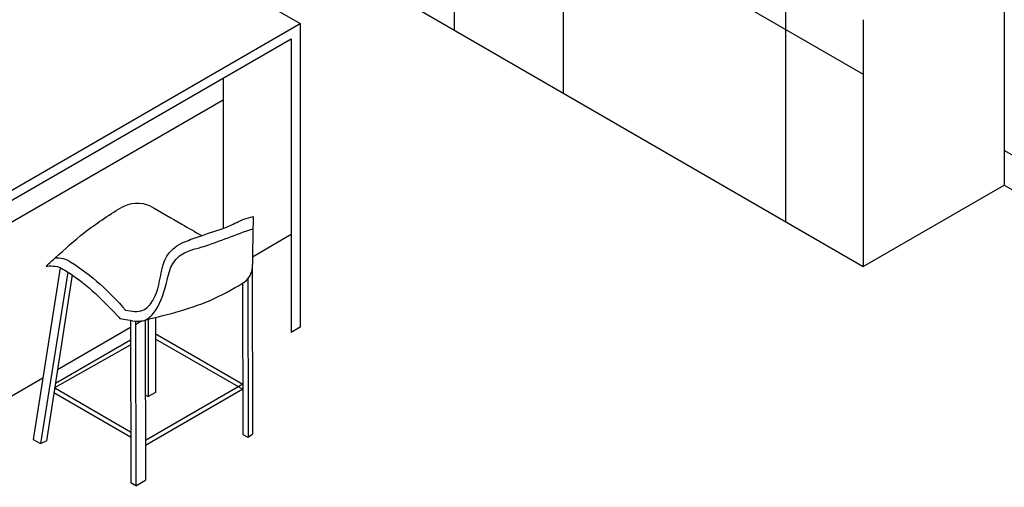
# Model space of a CAD drawing. Units: inches. Extents: x 5770 to 11891, y 3254 to 6808.
# Tile 5 of 15: x 5976 to 6073, y 3357 to 3403. Entities that reach past the tile are written whole.
import ezdxf

# ---------------------------------------------------------------- set-up
doc = ezdxf.new("R2010")
doc.units = ezdxf.units.IN
doc.layers.add('A-DOOR', color=4, linetype='Continuous', lineweight=25)
doc.layers.add('A-FURN', color=8, linetype='Continuous', lineweight=25)

# ---------------------------------------------------------------- blocks, each defined once
blk = doc.blocks.new('CHAIR')
for p, q in [((5928.223, 3348.403), (5925.543, 3331.45)), ((5928.971, 3347.97), (5926.273, 3331.028)), ((5929.389, 3347.696), (5926.875, 3331.298)), ((5947.206, 3348.302), (5947.238, 3331.95)), ((5946.251, 3346.874), (5946.28, 3331.945)), ((5946.776, 3347.308), (5946.806, 3331.701)), ((5935.159, 3343.206), (5935.191, 3327.159)), ((5935.654, 3343.133), (5935.686, 3326.874)), ((5936.612, 3343.231), (5936.643, 3327.426)), ((5936.929, 3343.309), (5936.929, 3335.675)), ((5937.628, 3343.481), (5937.628, 3336.079)), ((5937.622, 3341.892), (5946.27, 3336.899)), ((5927.681, 3336.559), (5935.163, 3340.783)), ((5927.752, 3337.017), (5935.163, 3341.283)), ((5937.622, 3341.392), (5946.27, 3336.399)), ((5946.27, 3336.899), (5936.636, 3331.337)), ((5935.182, 3331.676), (5927.604, 3336.052)), ((5935.181, 3332.177), (5927.674, 3336.511)), ((5936.627, 3335.849), (5936.929, 3335.675)), ((5946.27, 3336.399), (5936.636, 3330.837)), ((5937.628, 3336.079), (5936.929, 3335.675)), ((5946.28, 3331.945), (5946.754, 3331.671)), ((5946.754, 3331.671), (5947.238, 3331.95)), ((5925.543, 3331.45), (5926.273, 3331.028)), ((5926.273, 3331.028), (5926.875, 3331.298)), ((5935.686, 3326.874), (5935.191, 3327.159)), ((5935.686, 3326.874), (5936.643, 3327.426))]:
    blk.add_line(p, q)
blk.add_arc((5935.851, 3351.356), 3.391, 67.73594, 118.77676)
for points, knots in [([(5926.847, 3348.569), (5927.143, 3348.838), (5927.44, 3349.108), (5927.736, 3349.378), (5928.675, 3350.232), (5930.694, 3352.068), (5932.975, 3353.56), (5934.218, 3354.329)], [-1.200535, -1.200535, -1.200535, -1.200535, 0, 0, 0, 3.797995, 8.17369, 8.17369, 8.17369, 8.17369]), ([(5937.136, 3354.495), (5938.172, 3353.896), (5939.858, 3352.923), (5941.544, 3351.95), (5942.194, 3351.574)], [1.567957, 1.567957, 1.567957, 1.567957, 5.157778, 7.408601, 7.408601, 7.408601, 7.408601]), ([(5940.889, 3351.105), (5941.409, 3351.297), (5942.756, 3351.795), (5944.665, 3352.299), (5946.171, 3353.173), (5946.99, 3353.379), (5947.296, 3353.456)], [0, 0, 0, 0, 1.664278, 4.310629, 5.889247, 6.833724, 6.833724, 6.833724, 6.833724]), ([(5947.296, 3353.456), (5947.279, 3352.494), (5947.263, 3351.532), (5947.246, 3350.57), (5947.239, 3350.197), (5947.233, 3349.825), (5947.226, 3349.453), (5947.22, 3349.069), (5947.213, 3348.686), (5947.206, 3348.302)], [0, 0, 0, 0, 2.886502, 2.886502, 2.886502, 4.003886, 4.003886, 4.003886, 5.15459, 5.15459, 5.15459, 5.15459]), ([(5934.116, 3343.398), (5934.384, 3343.348), (5934.652, 3343.298), (5934.919, 3343.248), (5935.52, 3343.137), (5936.611, 3342.934), (5938.157, 3344.683), (5938.85, 3347.349), (5939.301, 3349.501), (5941.12, 3350.132), (5941.468, 3350.253), (5941.874, 3350.354), (5942.281, 3350.456), (5944.024, 3351.009), (5945.631, 3351.73), (5947.275, 3352.246)], [-0.758098, -0.758098, -0.758098, -0.758098, 0, 0, 0, 1.699756, 3.089131, 6.324639, 10.056959, 10.056959, 10.056959, 10.772274, 10.772274, 10.772274, 13.697346, 13.697346, 13.697346, 13.697346]), ([(5934.688, 3344.221), (5935.289, 3344.11), (5936.38, 3343.907), (5937.926, 3345.656), (5938.131, 3348.585), (5939.07, 3350.474), (5940.889, 3351.105)], [0, 0, 0, 0, 1.699756, 3.089131, 6.324639, 10.056959, 10.056959, 10.056959, 10.056959]), ([(5926.847, 3348.569), (5926.946, 3348.569), (5927.046, 3348.57), (5927.145, 3348.571), (5927.404, 3348.573), (5927.952, 3348.578), (5930.422, 3347.16), (5932.255, 3345.421), (5933.779, 3343.764), (5933.784, 3343.759), (5933.788, 3343.754), (5933.793, 3343.749), (5933.901, 3343.632), (5934.008, 3343.515), (5934.116, 3343.398)], [-0.293735, -0.293735, -0.293735, -0.293735, 0, 0, 0, 0.763361, 1.613257, 8.34273, 8.34273, 8.34273, 8.363036, 8.363036, 8.363036, 8.838355, 8.838355, 8.838355, 8.838355]), ([(5927.736, 3349.378), (5927.995, 3349.38), (5928.543, 3349.385), (5931.152, 3347.887), (5933.072, 3346.01), (5934.688, 3344.221)], [0, 0, 0, 0, 0.763361, 1.613257, 8.813397, 8.813397, 8.813397, 8.813397]), ([(5946.615, 3347.095), (5946.795, 3347.33), (5947.077, 3347.697), (5947.177, 3348.14), (5947.206, 3348.302)], [0, 0, 0, 0, 0.871891, 1.360739, 1.360739, 1.360739, 1.360739]), ([(5936.616, 3343.233), (5938.951, 3343.804), (5942.469, 3344.664), (5945.58, 3346.463), (5946.615, 3347.095)], [0, 0, 0, 0, 7.14919, 10.770772, 10.770772, 10.770772, 10.770772])]:
    blk.add_open_spline(points, degree=3, knots=knots)

msp = doc.modelspace()

# ---------------------------------------------------------------- linework, layer by layer
at = {"layer": 'A-DOOR'}
for p, q in [((6073.257, 3462.723), (6073.257, 3386.42)), ((6074.989, 3388.825), (6073.257, 3389.825)), ((6073.257, 3386.42), (6080.711, 3382.116))]:
    msp.add_line(p, q, dxfattribs=at)
at = {"layer": 'A-FURN'}
for p, q in [((5979.292, 3443.56), (6059.32, 3397.356)), ((5964.711, 3432.996), (6059.32, 3378.374)), ((5967.262, 3423.368), (6003.635, 3402.368)), ((6018.855, 3420.735), (6018.855, 3401.753)), ((6029.662, 3419.864), (6029.662, 3395.496)), ((6051.621, 3407.186), (6051.621, 3382.819)), ((5920.496, 3354.368), (6003.635, 3402.368)), ((6003.635, 3402.368), (6003.635, 3372.368)), ((6059.32, 3402.741), (6059.32, 3378.374)), ((5921.362, 3353.868), (6002.769, 3400.868)), ((6002.769, 3400.868), (6002.769, 3371.868)), ((5996.03, 3396.977), (5996.03, 3382.122)), ((5922.464, 3352.365), (5996.03, 3394.839)), ((6059.32, 3378.374), (6073.257, 3386.42)), ((6002.769, 3381.52), (5998.931, 3379.304)), ((5988.002, 3372.994), (5987.359, 3372.623)), ((5986.865, 3372.338), (5979.657, 3368.176)), ((6003.635, 3372.368), (6002.769, 3371.868)), ((5978.201, 3367.336), (5973.036, 3364.354))]:
    msp.add_line(p, q, dxfattribs=at)

# ---------------------------------------------------------------- block references
msp.add_blockref('CHAIR', (51.704, 29.852), dxfattribs=at)

doc.saveas('drawing.dxf')
